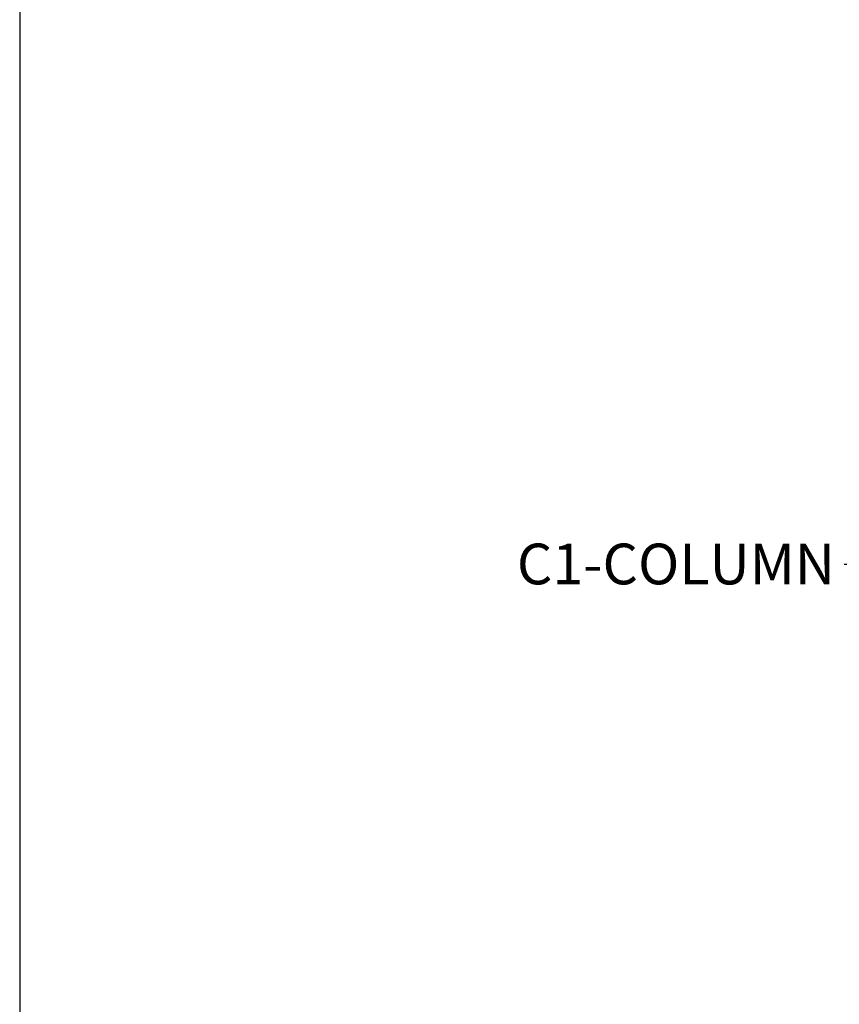
# Model space of a CAD drawing. Units: millimetres. Extents: x 20768 to 23556, y 50760 to 52704.
# Tile 2 of 36: x 20768 to 20949, y 51066 to 51283. Entities that reach past the tile are written whole.
import ezdxf
from ezdxf import colors
from ezdxf.entities.mleader import LeaderData, LeaderLine
from ezdxf.math import Vec2, Vec3

# ---------------------------------------------------------------- set-up
doc = ezdxf.new("R2010")
doc.units = ezdxf.units.MM
for name, color, linetype, lineweight in [('A-ANNO-TEXT', 7, 'Continuous', 18), ('A-ELEV', 7, 'Continuous', 25), ('A-ELEV-PATT', 8, 'Continuous', 13)]:
    doc.layers.add(name, color=color, linetype=linetype, lineweight=lineweight)
doc.styles.get("Standard").update_dxf_attribs({"font": 'arial.ttf'})

msp = doc.modelspace()

# ---------------------------------------------------------------- hatches: boundary and pattern name
at = {"layer": 'A-ELEV-PATT'}
h = msp.add_hatch(dxfattribs=at)
h.set_pattern_fill('AR-CONC', color=256, scale=8)
h.paths.add_polyline_path([(21106.86, 51149.66), (21094.86, 51149.66), (21094.86, 51077.66), (21022.86, 51077.66), (21022.86, 51149.66), (21016.86, 51149.66), (21016.86, 51077.66), (20866.86, 51077.66), (20866.86, 50768.86), (20854.86, 50768.86), (20854.86, 50759.86), (20890.86, 50759.86), (20890.86, 50768.86), (20878.86, 50768.86), (20878.86, 50807.86), (21016.86, 50807.86), (21016.86, 50768.86), (21007.86, 50768.86), (21007.86, 50759.86), (21031.86, 50759.86), (21031.86, 50768.86), (21022.86, 50768.86), (21022.86, 50807.86), (21094.86, 50807.86), (21094.86, 50768.86), (21082.86, 50768.86), (21082.86, 50759.86), (21118.86, 50759.86), (21118.86, 50768.86), (21106.86, 50768.86)])
h.paths.add_polyline_path([(21022.86, 50939.76), (21094.86, 50939.76), (21094.86, 50813.86), (21022.86, 50813.86)], flags=16)
h.paths.add_polyline_path([(21016.86, 50939.76), (21016.86, 50813.86), (20878.86, 50813.86), (20878.86, 50939.76)], flags=16)
h.paths.add_polyline_path([(21022.86, 50945.76), (21022.86, 51071.66), (21094.86, 51071.66), (21094.86, 50945.76)], flags=16)
h.paths.add_polyline_path([(21016.86, 50945.76), (20878.86, 50945.76), (20878.86, 51071.66), (21016.86, 51071.66)], flags=16)
h.paths.add_polyline_path([(20957.01, 51017.76), (20957.01, 51020.76), (21012.86, 51020.76), (21012.86, 51017.76)], flags=0)
h.paths.add_polyline_path([(21005.86, 50980.26), (20984.86, 50945.76), (20963.86, 50980.26), (20963.86, 51014.76), (21005.86, 51014.76)], flags=0)
h.paths.add_polyline_path([(20963.86, 50980.26), (20984.86, 51014.76), (21005.86, 50980.26)], flags=0)
h.paths.add_polyline_path([(21030.86, 50980.26), (21030.86, 51027.36), (21061.56, 51027.36), (21061.56, 50980.26)], flags=0)
h.paths.add_polyline_path([(21032.86, 50982.26), (21032.86, 51010.26), (21059.56, 51010.26), (21059.56, 50982.26)], flags=0)
h.paths.add_polyline_path([(21034.86, 50984.26), (21034.86, 51008.26), (21045.21, 51008.26), (21045.21, 50984.26)], flags=0)
h.paths.add_polyline_path([(21030.86, 50895.46), (21061.56, 50895.46), (21061.56, 50848.36), (21030.86, 50848.36)], flags=0)
h.paths.add_polyline_path([(21032.86, 50893.46), (21059.56, 50893.46), (21059.56, 50880.36), (21032.86, 50880.36)], flags=0)
h.paths.add_polyline_path([(21047.21, 50984.26), (21047.21, 51008.26), (21057.56, 51008.26), (21057.56, 50984.26)], flags=0)
h.paths.add_polyline_path([(20989.07, 50982.94), (20988.43, 50982.94, -0.960515), (20986.68, 50983.01, -0.414214), (20987.56, 50983.89), (20987.56, 50984.45, -0.357901), (20987.34, 50984.72, -1), (20987.88, 50984.72, -0.34824), (20987.67, 50984.45), (20987.67, 50983.88, -0.376216), (20988.43, 50983.01), (20989.07, 50983.01)], flags=0)
h.paths.add_polyline_path([(21012.86, 50888.86), (21012.86, 50885.86), (20957.01, 50885.86), (20957.01, 50888.86)], flags=0)
h.paths.add_polyline_path([(20981.29, 50982.94), (20980.65, 50982.94), (20980.65, 50983.01), (20981.28, 50983.01, -0.376216), (20982.04, 50983.88), (20982.04, 50984.45, -0.34824), (20981.83, 50984.72, -1), (20982.38, 50984.72, -0.357901), (20982.16, 50984.45), (20982.16, 50983.89, -0.414214), (20983.04, 50983.01, -0.960515)], flags=0)
h.paths.add_polyline_path([(21005.86, 50882.86), (21005.86, 50848.36), (20984.86, 50813.86), (20963.86, 50848.36), (20963.86, 50882.86)], flags=0)
h.paths.add_polyline_path([(21032.86, 50878.36), (21059.56, 50878.36), (21059.56, 50850.36), (21032.86, 50850.36)], flags=0)
h.paths.add_polyline_path([(21034.86, 50876.36), (21045.21, 50876.36), (21045.21, 50852.36), (21034.86, 50852.36)], flags=0)
h.paths.add_polyline_path([(20984.86, 50882.86), (21005.86, 50848.36), (20963.86, 50848.36)], flags=0)
h.paths.add_polyline_path([(20950.86, 50825.86), (20914.86, 50825.86), (20914.86, 50873.86), (20950.86, 50873.86)], flags=0)
h.paths.add_polyline_path([(20950.86, 50957.76), (20914.86, 50957.76), (20914.86, 51005.76), (20950.86, 51005.76)], flags=0)
h.paths.add_polyline_path([(21047.21, 50876.36), (21057.56, 50876.36), (21057.56, 50852.36), (21047.21, 50852.36)], flags=0)
h.paths.add_polyline_path([(21032.86, 51012.26), (21032.86, 51025.36), (21059.56, 51025.36), (21059.56, 51012.26)], flags=0)
h.paths.add_polyline_path([(20987.88, 50852.82, -0.34824), (20987.67, 50852.55), (20987.67, 50851.98, -0.376216), (20988.43, 50851.11), (20989.07, 50851.11), (20989.07, 50851.04), (20988.43, 50851.04, -0.960515), (20986.68, 50851.11, -0.414214), (20987.56, 50851.99), (20987.56, 50852.55, -0.357901), (20987.34, 50852.82, -1)], flags=0)
h.paths.add_polyline_path([(20982.38, 50852.82, -0.357901), (20982.16, 50852.55), (20982.16, 50851.99, -0.414214), (20983.04, 50851.11, -0.960515), (20981.29, 50851.04), (20980.65, 50851.04), (20980.65, 50851.11), (20981.28, 50851.11, -0.376216), (20982.04, 50851.98), (20982.04, 50852.55, -0.34824), (20981.83, 50852.82, -1)], flags=0)

# ---------------------------------------------------------------- linework, layer by layer
at = {"layer": 'A-ELEV'}
msp.add_line((20768.14, 51623.53), (20768.14, 50975.78), dxfattribs=at)

# ---------------------------------------------------------------- leaders
at = {"layer": 'A-ANNO-TEXT'}
ml = msp.add_multileader_mtext('Standard', dxfattribs=at)
ml.set_content('C1-COLUMN', color=256)
ml.set_leader_properties()
ml.build(insert=Vec2(0, 0))
ctx = ml.context
ctx.base_point, ctx.char_height, ctx.plane_origin = Vec3(20873.04, 51163.09), 9, Vec3(20977.17, 51163.09)
ctx.text_align_type = 2
notes = []
notes.append((ctx, [(0, (1, 1, 0), (20958.12, 51163.09), (-1, 0), 8, [(0, [(20977.17, 51163.09)], 0, [])])]))
ctx.mtext.insert, ctx.mtext.alignment, ctx.mtext.flow_direction = Vec3(20948.12, 51167.67), 3, 5
for ctx, leaders in notes:
    for number, flags, end, landing, length, lines in leaders:
        leader = LeaderData()
        leader.index, (leader.has_last_leader_line, leader.has_dogleg_vector, leader.attachment_direction) = number, flags
        leader.last_leader_point, leader.dogleg_vector, leader.dogleg_length = Vec3(end), Vec3(landing), length
        for number, points, colour, breaks in lines:
            line = LeaderLine()
            line.index, line.vertices, line.color, line.breaks = number, Vec3.list(points), colors.encode_raw_color(colour), breaks
            leader.lines.append(line)
        ctx.leaders.append(leader)

doc.saveas('drawing.dxf')
